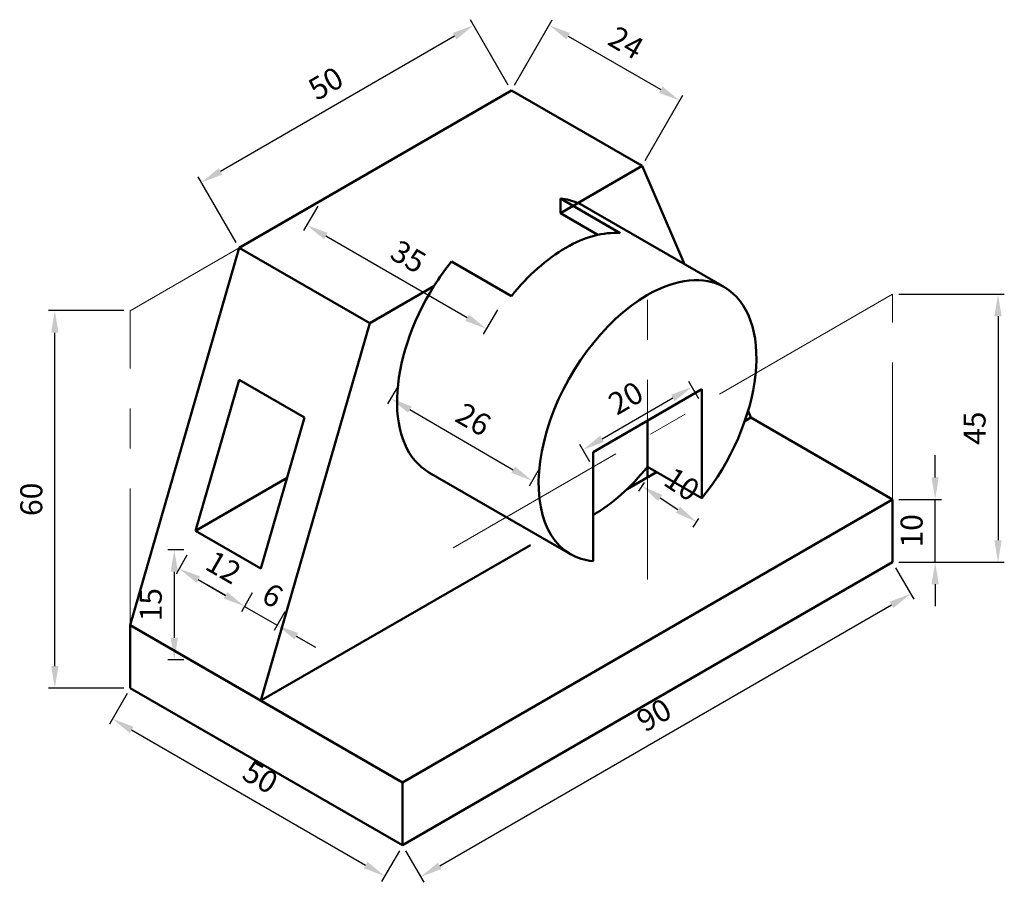
# Model space of a CAD drawing. Units: millimetres. Extents: x 2878 to 3035, y 958 to 1095.
import ezdxf

# ---------------------------------------------------------------- set-up
doc = ezdxf.new("R2010")
doc.units = ezdxf.units.MM
doc.linetypes.add('CENTER', pattern=[50.8, 31.75, -6.35, 6.35, -6.35])
for name, color, linetype, lineweight in [('M-CNTR', 4, 'CENTER', 18), ('M-CONS', 8, 'CENTER', 13), ('M-DIMS', 3, 'Continuous', 25), ('M-OUTL', 7, 'Continuous', 50)]:
    doc.layers.add(name, color=color, linetype=linetype, lineweight=lineweight)
doc.styles.get("Standard").update_dxf_attribs({"font": 'arial.ttf'})
doc.dimstyles.new('AM_ISO$0', dxfattribs={"dimtxt": 3.5, "dimasz": 3.5, "dimexe": 1, "dimexo": 1, "dimgap": 1.5, "dimtad": 1, "dimdsep": 46, "dimtxsty": 'Standard', "dimcen": 0, "dimclrd": 256, "dimclre": 256, "dimclrt": 2, "dimadec": 0, "dimazin": 2, "dimtp": 0.1, "dimtm": 0.1, "dimtfac": 0.71, "dimtdec": 3, "dimtmove": 0, "dimatfit": 3, "dimfxl": 1, "dimlwd": -1, "dimlwe": -1, "dimarcsym": 1})

# ---------------------------------------------------------------- blocks, each defined once
blk = doc.blocks.new('*D3')
at = {"layer": 'Defpoints', "color": 0, "transparency": 16777216}
for p in [(3016.76, 1008.94), (3019.65, 1003.93), (2938.82, 963.94)]:
    blk.add_point(p, dxfattribs=at)
at = {"layer": 'M-DIMS', "color": 0, "linetype": 'ByBlock', "transparency": 16777216}
for p, q in [((3017.26, 1008.07), (3020.15, 1003.06)), ((2944.74, 960.68), (3016.62, 1002.18)), ((2939.32, 963.07), (2942.21, 958.06))]:
    blk.add_line(p, q, dxfattribs=at)
at = {"layer": 'M-DIMS', "color": 0, "transparency": 16777216}
for points in [[(3016.33, 1002.68), (3016.91, 1001.67), (3019.65, 1003.93)], [(2944.45, 961.18), (2945.03, 960.17), (2941.71, 958.93)]]:
    blk.add_solid(points, dxfattribs=at)
at = {"layer": 'M-DIMS', "color": 0, "transparency": 16777216, "insert": (2979.04, 984.27), "char_height": 3.5, "attachment_point": 5, "rotation": 30}
blk.add_mtext('90', dxfattribs=at)
blk = doc.blocks.new('*D4')
at = {"layer": 'Defpoints', "color": 0, "transparency": 16777216}
for p in [(3016.76, 1018.94), (3023.54, 1018.94), (3016.76, 1008.94)]:
    blk.add_point(p, dxfattribs=at)
at = {"layer": 'M-DIMS', "color": 0, "linetype": 'ByBlock', "transparency": 16777216}
for p, q in [((3023.54, 1022.44), (3023.54, 1025.94)), ((3017.76, 1018.94), (3024.54, 1018.94)), ((3023.54, 1008.94), (3023.54, 1018.94)), ((3017.76, 1008.94), (3024.54, 1008.94)), ((3023.54, 1005.44), (3023.54, 1001.94))]:
    blk.add_line(p, q, dxfattribs=at)
at = {"layer": 'M-DIMS', "color": 0, "transparency": 16777216}
for points in [[(3022.96, 1022.44), (3024.12, 1022.44), (3023.54, 1018.94)], [(3022.96, 1005.44), (3024.12, 1005.44), (3023.54, 1008.94)]]:
    blk.add_solid(points, dxfattribs=at)
at = {"layer": 'M-DIMS', "color": 0, "transparency": 16777216, "insert": (3020.25, 1013.94), "char_height": 3.5, "attachment_point": 5, "rotation": 90}
blk.add_mtext('10', dxfattribs=at)
blk = doc.blocks.new('*D5')
at = {"layer": 'Defpoints', "color": 0, "transparency": 16777216}
for p in [(3016.76, 1051.55), (3016.76, 1008.94), (3033.54, 1008.94)]:
    blk.add_point(p, dxfattribs=at)
at = {"layer": 'M-DIMS', "color": 0, "linetype": 'ByBlock', "transparency": 16777216}
for p, q in [((3017.76, 1051.55), (3034.54, 1051.55)), ((3033.54, 1048.05), (3033.54, 1012.44)), ((3017.76, 1008.94), (3034.54, 1008.94))]:
    blk.add_line(p, q, dxfattribs=at)
at = {"layer": 'M-DIMS', "color": 0, "transparency": 16777216}
for points in [[(3032.96, 1048.05), (3034.12, 1048.05), (3033.54, 1051.55)], [(3032.96, 1012.44), (3034.12, 1012.44), (3033.54, 1008.94)]]:
    blk.add_solid(points, dxfattribs=at)
at = {"layer": 'M-DIMS', "color": 0, "transparency": 16777216, "insert": (3030.26, 1030.25), "char_height": 3.5, "attachment_point": 5, "rotation": 90}
blk.add_mtext('45', dxfattribs=at)
blk = doc.blocks.new('*D6')
at = {"layer": 'Defpoints', "color": 0, "transparency": 16777216}
for p in [(2956.14, 1083.94), (2982.92, 1082.33), (2976.92, 1071.94)]:
    blk.add_point(p, dxfattribs=at)
at = {"layer": 'M-DIMS', "color": 0, "linetype": 'ByBlock', "transparency": 16777216}
for p, q in [((2956.64, 1084.8), (2962.64, 1095.2)), ((2965.17, 1092.58), (2979.89, 1084.08)), ((2977.42, 1072.8), (2983.42, 1083.2))]:
    blk.add_line(p, q, dxfattribs=at)
at = {"layer": 'M-DIMS', "color": 0, "transparency": 16777216}
for points in [[(2965.46, 1093.08), (2964.88, 1092.07), (2962.14, 1094.33)], [(2980.18, 1084.58), (2979.6, 1083.57), (2982.92, 1082.33)]]:
    blk.add_solid(points, dxfattribs=at)
at = {"layer": 'M-DIMS', "color": 0, "transparency": 16777216, "insert": (2974.16, 1091.15), "char_height": 3.5, "attachment_point": 5, "rotation": 330}
blk.add_mtext('24', dxfattribs=at)
blk = doc.blocks.new('*D7')
at = {"layer": 'Defpoints', "color": 0, "transparency": 16777216}
for p in [(2956.14, 1083.94), (2906.84, 1069.33), (2912.84, 1058.94)]:
    blk.add_point(p, dxfattribs=at)
at = {"layer": 'M-DIMS', "color": 0, "linetype": 'ByBlock', "transparency": 16777216}
for p, q in [((2955.64, 1084.8), (2949.64, 1095.2)), ((2947.11, 1092.58), (2909.87, 1071.08)), ((2912.34, 1059.8), (2906.34, 1070.2))]:
    blk.add_line(p, q, dxfattribs=at)
at = {"layer": 'M-DIMS', "color": 0, "transparency": 16777216}
for points in [[(2946.81, 1093.08), (2947.4, 1092.07), (2950.14, 1094.33)], [(2909.58, 1071.58), (2910.16, 1070.57), (2906.84, 1069.33)]]:
    blk.add_solid(points, dxfattribs=at)
at = {"layer": 'M-DIMS', "color": 0, "transparency": 16777216, "insert": (2926.84, 1084.68), "char_height": 3.5, "attachment_point": 5, "rotation": 30}
blk.add_mtext('50', dxfattribs=at)
blk = doc.blocks.new('*D8')
at = {"layer": 'Defpoints', "color": 0, "transparency": 16777216}
for p in [(2938.58, 1037.75), (2961.08, 1024.66), (2959.46, 1021.89)]:
    blk.add_point(p, dxfattribs=at)
at = {"layer": 'M-DIMS', "color": 0, "linetype": 'ByBlock', "transparency": 16777216}
for p, q in [((2938.07, 1036.88), (2936.46, 1034.11)), ((2939.99, 1033.21), (2956.44, 1023.65)), ((2960.57, 1023.8), (2958.96, 1021.02))]:
    blk.add_line(p, q, dxfattribs=at)
at = {"layer": 'M-DIMS', "color": 0, "transparency": 16777216}
for points in [[(2940.28, 1033.72), (2939.7, 1032.71), (2936.96, 1034.97)], [(2956.73, 1024.15), (2956.14, 1023.14), (2959.46, 1021.89)]]:
    blk.add_solid(points, dxfattribs=at)
at = {"layer": 'M-DIMS', "color": 0, "transparency": 16777216, "insert": (2949.87, 1031.27), "char_height": 3.5, "attachment_point": 5, "rotation": 329.8135}
blk.add_mtext('26', dxfattribs=at)
blk = doc.blocks.new('*D9')
at = {"layer": 'Defpoints', "color": 0, "transparency": 16777216}
for p in [(2984.85, 1036.81), (2986.45, 1034.05), (2969.13, 1024.05)]:
    blk.add_point(p, dxfattribs=at)
at = {"layer": 'M-DIMS', "color": 0, "linetype": 'ByBlock', "transparency": 16777216}
for p, q in [((2985.95, 1034.92), (2984.35, 1037.68)), ((2970.57, 1028.56), (2981.82, 1035.06)), ((2968.63, 1024.92), (2967.03, 1027.68))]:
    blk.add_line(p, q, dxfattribs=at)
at = {"layer": 'M-DIMS', "color": 0, "transparency": 16777216}
for points in [[(2981.53, 1035.57), (2982.12, 1034.56), (2984.85, 1036.81)], [(2970.27, 1029.07), (2970.86, 1028.06), (2967.53, 1026.81)]]:
    blk.add_solid(points, dxfattribs=at)
at = {"layer": 'M-DIMS', "color": 0, "transparency": 16777216, "insert": (2974.55, 1034.66), "char_height": 3.5, "attachment_point": 5, "rotation": 30}
blk.add_mtext('20', dxfattribs=at)
blk = doc.blocks.new('*D10')
at = {"layer": 'Defpoints', "color": 0, "transparency": 16777216}
for p in [(2977.79, 1022.44), (2976.89, 1021.07), (2986.45, 1016.73)]:
    blk.add_point(p, dxfattribs=at)
at = {"layer": 'M-DIMS', "color": 0, "linetype": 'ByBlock', "transparency": 16777216}
for p, q in [((2977.24, 1021.6), (2976.34, 1020.24)), ((2982.63, 1017.29), (2979.81, 1019.15)), ((2985.9, 1015.9), (2985, 1014.53))]:
    blk.add_line(p, q, dxfattribs=at)
at = {"layer": 'M-DIMS', "color": 0, "transparency": 16777216}
for points in [[(2980.13, 1019.64), (2979.49, 1018.66), (2976.89, 1021.07)], [(2982.95, 1017.78), (2982.31, 1016.81), (2985.55, 1015.37)]]:
    blk.add_solid(points, dxfattribs=at)
at = {"layer": 'M-DIMS', "color": 0, "transparency": 16777216, "insert": (2983.03, 1020.97), "char_height": 3.5, "attachment_point": 5, "rotation": 326.6284}
blk.add_mtext('10', dxfattribs=at)
blk = doc.blocks.new('*D11')
at = {"layer": 'Defpoints', "color": 0, "transparency": 16777216}
for p in [(2925.83, 1066.44), (2923.58, 1062.55), (2954.41, 1049.94)]:
    blk.add_point(p, dxfattribs=at)
at = {"layer": 'M-DIMS', "color": 0, "linetype": 'ByBlock', "transparency": 16777216}
for p, q in [((2925.33, 1065.57), (2923.08, 1061.69)), ((2949.13, 1047.8), (2926.61, 1060.8)), ((2953.91, 1049.07), (2951.66, 1045.19))]:
    blk.add_line(p, q, dxfattribs=at)
at = {"layer": 'M-DIMS', "color": 0, "transparency": 16777216}
for points in [[(2926.91, 1061.31), (2926.32, 1060.3), (2923.58, 1062.55)], [(2949.42, 1048.31), (2948.84, 1047.3), (2952.16, 1046.05)]]:
    blk.add_solid(points, dxfattribs=at)
at = {"layer": 'M-DIMS', "color": 0, "transparency": 16777216, "insert": (2939.52, 1057.15), "char_height": 3.5, "attachment_point": 5, "rotation": 330}
blk.add_mtext('35', dxfattribs=at)
blk = doc.blocks.new('*D12')
at = {"layer": 'Defpoints', "color": 0, "transparency": 16777216}
for p in [(2883.52, 1048.94), (2895.52, 1048.94), (2895.52, 988.94)]:
    blk.add_point(p, dxfattribs=at)
at = {"layer": 'M-DIMS', "color": 0, "linetype": 'ByBlock', "transparency": 16777216}
for p, q in [((2894.52, 1048.94), (2882.52, 1048.94)), ((2883.52, 992.44), (2883.52, 1045.44)), ((2894.52, 988.94), (2882.52, 988.94))]:
    blk.add_line(p, q, dxfattribs=at)
at = {"layer": 'M-DIMS', "color": 0, "transparency": 16777216}
for points in [[(2882.93, 1045.44), (2884.1, 1045.44), (2883.52, 1048.94)], [(2882.93, 992.44), (2884.1, 992.44), (2883.52, 988.94)]]:
    blk.add_solid(points, dxfattribs=at)
at = {"layer": 'M-DIMS', "color": 0, "transparency": 16777216, "insert": (2880.23, 1018.94), "char_height": 3.5, "attachment_point": 5, "rotation": 90}
blk.add_mtext('60', dxfattribs=at)
blk = doc.blocks.new('*D13')
at = {"layer": 'Defpoints', "color": 0, "transparency": 16777216}
for p in [(2895.52, 988.94), (2938.82, 963.94), (2935.99, 959.05)]:
    blk.add_point(p, dxfattribs=at)
at = {"layer": 'M-DIMS', "color": 0, "linetype": 'ByBlock', "transparency": 16777216}
for p, q in [((2895.02, 988.07), (2892.19, 983.18)), ((2895.72, 982.3), (2932.96, 960.8)), ((2938.32, 963.07), (2935.49, 958.18))]:
    blk.add_line(p, q, dxfattribs=at)
at = {"layer": 'M-DIMS', "color": 0, "transparency": 16777216}
for points in [[(2896.02, 982.8), (2895.43, 981.79), (2892.69, 984.05)], [(2933.26, 961.3), (2932.67, 960.29), (2935.99, 959.05)]]:
    blk.add_solid(points, dxfattribs=at)
at = {"layer": 'M-DIMS', "color": 0, "transparency": 16777216, "insert": (2915.99, 974.4), "char_height": 3.5, "attachment_point": 5, "rotation": 330}
blk.add_mtext('50', dxfattribs=at)
blk = doc.blocks.new('*D14')
at = {"layer": 'Defpoints', "color": 0, "transparency": 16777216}
for p in [(2905.04, 1010.94), (2915.43, 1004.94), (2913.7, 1001.93)]:
    blk.add_point(p, dxfattribs=at)
at = {"layer": 'M-DIMS', "color": 0, "linetype": 'ByBlock', "transparency": 16777216}
for p, q in [((2904.54, 1010.07), (2902.81, 1007.07)), ((2906.34, 1006.18), (2910.67, 1003.68)), ((2914.93, 1004.07), (2913.2, 1001.07))]:
    blk.add_line(p, q, dxfattribs=at)
at = {"layer": 'M-DIMS', "color": 0, "transparency": 16777216}
for points in [[(2906.63, 1006.69), (2906.05, 1005.68), (2903.31, 1007.93)], [(2910.96, 1004.19), (2910.38, 1003.18), (2913.7, 1001.93)]]:
    blk.add_solid(points, dxfattribs=at)
at = {"layer": 'M-DIMS', "color": 0, "transparency": 16777216, "insert": (2910.13, 1007.75), "char_height": 3.5, "attachment_point": 5, "rotation": 330}
blk.add_mtext('12', dxfattribs=at)
blk = doc.blocks.new('*D15')
at = {"layer": 'Defpoints', "color": 0, "transparency": 16777216}
for p in [(2915.43, 1004.94), (2920.63, 1001.94), (2918.9, 998.93)]:
    blk.add_point(p, dxfattribs=at)
at = {"layer": 'M-DIMS', "color": 0, "linetype": 'ByBlock', "transparency": 16777216}
for p, q in [((2910.67, 1003.68), (2907.64, 1005.43)), ((2914.93, 1004.07), (2913.2, 1001.07)), ((2913.7, 1001.93), (2918.9, 998.93)), ((2920.13, 1001.07), (2918.4, 998.07)), ((2921.93, 997.18), (2924.96, 995.43))]:
    blk.add_line(p, q, dxfattribs=at)
at = {"layer": 'M-DIMS', "color": 0, "transparency": 16777216}
for points in [[(2910.96, 1004.19), (2910.38, 1003.18), (2913.7, 1001.93)], [(2922.22, 997.69), (2921.64, 996.68), (2918.9, 998.93)]]:
    blk.add_solid(points, dxfattribs=at)
at = {"layer": 'M-DIMS', "color": 0, "transparency": 16777216, "insert": (2917.94, 1003.28), "char_height": 3.5, "attachment_point": 5, "rotation": 330}
blk.add_mtext('6', dxfattribs=at)
blk = doc.blocks.new('*D16')
at = {"layer": 'Defpoints', "color": 0, "transparency": 16777216}
for p in [(2905.04, 1010.94), (2902.52, 993.44), (2905.04, 993.44)]:
    blk.add_point(p, dxfattribs=at)
at = {"layer": 'M-DIMS', "color": 0, "linetype": 'ByBlock', "transparency": 16777216}
for p, q in [((2904.04, 1010.94), (2901.52, 1010.94)), ((2902.52, 1007.44), (2902.52, 996.94)), ((2904.04, 993.44), (2901.52, 993.44))]:
    blk.add_line(p, q, dxfattribs=at)
at = {"layer": 'M-DIMS', "color": 0, "transparency": 16777216}
for points in [[(2901.94, 1007.44), (2903.11, 1007.44), (2902.52, 1010.94)], [(2901.94, 996.94), (2903.11, 996.94), (2902.52, 993.44)]]:
    blk.add_solid(points, dxfattribs=at)
at = {"layer": 'M-DIMS', "color": 0, "transparency": 16777216, "insert": (2899.24, 1002.19), "char_height": 3.5, "attachment_point": 5, "rotation": 90}
blk.add_mtext('15', dxfattribs=at)

msp = doc.modelspace()

# ---------------------------------------------------------------- linework, layer by layer
at = {"layer": 'M-CNTR'}
for p, q in [((2977.788, 1006.197), (2977.788, 1056.735)), ((3016.759, 1051.553), (2946.892, 1011.215))]:
    msp.add_line(p, q, dxfattribs=at)
at = {"layer": 'M-CONS'}
for p, q in [((2912.836, 1058.937), (2895.515, 1048.937)), ((3016.759, 1008.937), (3016.759, 1051.553)), ((2895.515, 988.937), (2895.515, 1048.937)), ((3016.759, 1008.937), (3016.759, 1018.937))]:
    msp.add_line(p, q, dxfattribs=at)
at = {"layer": 'M-OUTL'}
for p, q in [((2912.836, 1058.937), (2956.137, 1083.937)), ((2956.137, 1083.937), (2976.922, 1071.937)), ((2976.922, 1071.937), (2963.931, 1064.437)), ((2976.922, 1071.937), (2968.261, 1066.937)), ((2968.261, 1066.937), (2976.922, 1071.937)), ((2983.686, 1056.316), (2976.922, 1071.937)), ((2973.458, 1061.257), (2963.931, 1066.757)), ((2963.931, 1064.437), (2963.931, 1066.757)), ((2990.035, 1052.65), (2967.519, 1065.65)), ((2969.894, 1060.994), (2963.931, 1064.437)), ((2912.836, 1058.937), (2895.515, 998.937)), ((2933.62, 1046.937), (2912.836, 1058.937)), ((2956.137, 1051.257), (2946.611, 1056.757)), ((2943.815, 1052.823), (2933.62, 1046.937)), ((2933.62, 1046.937), (2942.281, 1051.937)), ((2933.62, 1046.937), (2942.281, 1051.937)), ((2933.62, 1046.937), (2916.3, 986.937)), ((2912.836, 1037.937), (2905.908, 1013.937)), ((2923.228, 1031.937), (2912.836, 1037.937)), ((2969.128, 1026.437), (2986.448, 1036.437)), ((2986.448, 1036.437), (2986.448, 1019.116)), ((2994.242, 1031.937), (2993.783, 1032.998)), ((2994.184, 1032.072), (2994.242, 1031.937)), ((2923.228, 1031.937), (2916.3, 1007.937)), ((2977.788, 1024.116), (2977.788, 1031.437)), ((2993.255, 1031.367), (2994.242, 1031.937)), ((2994.133, 1031.874), (2994.242, 1031.937)), ((2994.133, 1031.874), (2994.242, 1031.937)), ((2994.242, 1031.937), (3016.759, 1018.937)), ((2977.788, 1029.053), (2977.788, 1022.437)), ((2969.128, 1026.437), (2969.128, 1009.116)), ((2965.54, 1010.224), (2943.024, 1023.224)), ((2974.536, 1020.559), (2979.242, 1023.277)), ((2986.448, 1019.116), (2977.788, 1024.116)), ((2905.908, 1013.937), (2920.457, 1022.337)), ((2938.817, 973.937), (3016.759, 1018.937)), ((3016.759, 1018.937), (3016.759, 1008.937)), ((3016.759, 1008.937), (3016.759, 1018.937)), ((2916.3, 1007.937), (2905.908, 1013.937)), ((2916.3, 986.937), (2959.154, 1011.679)), ((2916.3, 986.937), (2959.154, 1011.679)), ((3016.759, 1008.937), (2938.817, 963.937)), ((2895.515, 988.937), (2895.515, 998.937)), ((2895.515, 998.937), (2938.817, 973.937)), ((2895.515, 998.937), (2916.3, 986.937)), ((2938.817, 963.937), (2895.515, 988.937)), ((2938.817, 973.937), (2938.817, 963.937))]:
    msp.add_line(p, q, dxfattribs=at)
for centre, start_param, end_param in [((2955.271, 1044.437), 0.0626639, 0.2617994), ((2955.271, 1044.437), 0, 0.0626639), ((2964.797, 1038.937), 0.2617994, 0.7853982), ((2964.797, 1038.937), 0.7853982, 1.3089969), ((2955.271, 1044.437), 1.3089969, 1.5081324), ((2977.788, 1031.437), 0, 0.7853982), ((2955.271, 1044.437), 1.5081324, 3.1415927), ((2977.788, 1031.437), 4.4505896, 6.2831853), ((2977.788, 1031.437), 0.7853982, 3.1415927), ((2969.128, 1036.437), 3.9269908, 4.4505896), ((2977.788, 1031.437), 3.1415927, 3.403392)]:
    msp.add_ellipse(centre, major_axis=(12.247, 21.213), ratio=0.5773503, start_param=start_param, end_param=end_param, dxfattribs=at)

# ---------------------------------------------------------------- dimensions: what is measured, and where the dimension line sits
at = {"layer": 'M-DIMS'}
for p1, p2, distance, override, picture, middle in [((2956.137, 1083.937), (2912.836, 1058.937), -12, {"dimclrd": 0, "dimclre": 0, "dimclrt": 0}, '*D7', (2926.843, 1084.676)), ((2956.137, 1083.937), (2976.922, 1071.937), 12, {"dimpost": '', "dimclrd": 0, "dimclre": 0, "dimclrt": 0}, '*D6', (2974.158, 1091.15)), ((2895.515, 988.937), (2895.515, 1048.937), 12, {"dimpost": '', "dimclrd": 0, "dimclre": 0, "dimclrt": 0}, '*D12', (2880.228, 1018.937)), ((2969.128, 1024.053), (2986.448, 1034.053), 3.186, {"dimclrd": 0, "dimclre": 0, "dimclrt": 0}, '*D9', (2974.551, 1034.659)), ((3016.759, 1008.937), (3016.759, 1018.937), -6.783, {"dimclrd": 0, "dimclre": 0, "dimclrt": 0}, '*D4', (3020.254, 1013.937)), ((2905.042, 1010.937), (2915.434, 1004.937), -3.469, {"dimclrd": 0, "dimclre": 0, "dimclrt": 0}, '*D14', (2910.132, 1007.754)), ((2938.817, 963.937), (3016.759, 1008.937), -5.786, {"dimpost": '', "dimclrd": 0, "dimclre": 0, "dimclrt": 0}, '*D3', (2979.037, 984.272)), ((2895.515, 988.937), (2938.817, 963.937), -5.643, {"dimpost": '', "dimclrd": 0, "dimclre": 0, "dimclrt": 0}, '*D13', (2915.988, 974.396))]:
    dim = msp.add_aligned_dim(p1=p1, p2=p2, distance=distance, dimstyle='AM_ISO$0', override=override, dxfattribs=at)
    dim.commit()
    dim.dimension.update_dxf_attribs({"geometry": picture, "text_midpoint": middle})
for p1, p2, distance, text, picture, middle in [((2954.405, 1049.937), (2925.826, 1066.437), 4.485, '35', '*D11', (2939.517, 1057.15)), ((2938.577, 1037.747), (2961.076, 1024.66), -3.207, '26', '*D8', (2949.867, 1031.272)), ((2986.448, 1016.733), (2977.788, 1022.437), 1.632, '10', '*D10', (2983.028, 1020.967)), ((2905.042, 1010.937), (2905.042, 993.437), -2.519, '15', '*D16', (2899.236, 1002.187))]:
    dim = msp.add_aligned_dim(p1=p1, p2=p2, distance=distance, text=text, dimstyle='AM_ISO$0', override={"dimpost": '', "dimclrd": 0, "dimclre": 0, "dimclrt": 0}, dxfattribs=at)
    dim.commit()
    dim.dimension.update_dxf_attribs({"geometry": picture, "text_midpoint": middle})
dim = msp.add_linear_dim(base=(3033.541, 1008.937), p1=(3016.759, 1051.553), p2=(3016.759, 1008.937), angle=90, text='45', dimstyle='AM_ISO$0', override={"dimpost": '', "dimclrd": 0, "dimclre": 0, "dimclrt": 0}, dxfattribs=at)
dim.commit()
dim.dimension.update_dxf_attribs({"geometry": '*D5', "text_midpoint": (3030.262, 1030.245)})
dim = msp.add_linear_dim(base=(2918.896, 998.933), p1=(2915.434, 1004.937), p2=(2920.63, 1001.937), angle=150, dimstyle='AM_ISO$0', override={"dimclrd": 0, "dimclre": 0, "dimclrt": 0}, dxfattribs=at)
dim.commit()
dim.dimension.update_dxf_attribs({"geometry": '*D15', "text_midpoint": (2917.941, 1003.279)})

doc.saveas('drawing.dxf')
